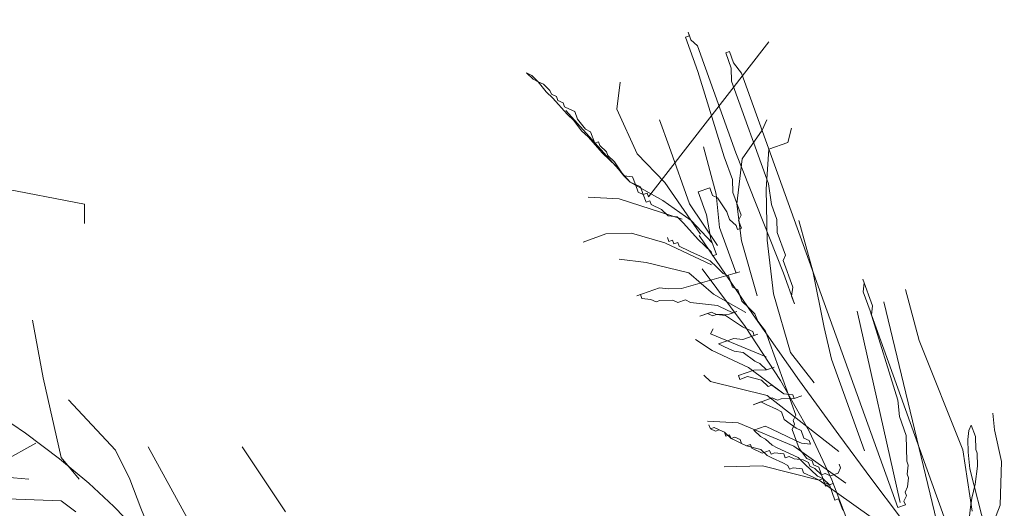
# Model space of a CAD drawing. Units: millimetres. Extents: x 595116 to 630915, y 909473 to 920225.
# Tile 23 of 134: x 629599.598 to 629606.562, y 919177.315 to 919180.767. Entities that reach past the tile are written whole.
import ezdxf

# ---------------------------------------------------------------- set-up
doc = ezdxf.new("R2010")
doc.units = ezdxf.units.MM
doc.layers.add('Dimension', color=3, linetype='Continuous', lineweight=18)
doc.layers.add('L-PLNT', color=85, linetype='Continuous', lineweight=13)
doc.styles.get("Standard").update_dxf_attribs({"font": 'arial.ttf'})
doc.dimstyles.new('ISO-25', dxfattribs={"dimtxt": 9, "dimasz": 6, "dimexe": 1.25, "dimexo": 0.625, "dimtad": 1, "dimlunit": 4, "dimtxsty": 'Standard', "dimcen": 2.5, "dimadec": 0, "dimazin": 0, "dimtfac": 1, "dimtmove": 0, "dimatfit": 3, "dimfxl": 1, "dimarcsym": 0})

# ---------------------------------------------------------------- blocks, each defined once
blk = doc.blocks.new('A$C143125F4')
for p, q in [((4.89065, 2.30713), (4.98365, 2.28921)), ((4.98365, 2.28921), (4.98365, 2.27577))]:
    blk.add_line(p, q)
blk = doc.blocks.new('A$C4FB75ABC')
for p, q in [((2.2354, 4.7176), (2.2283, 4.715)), ((2.2283, 4.715), (2.2515, 4.6504)), ((2.238, 4.7104), (2.2329, 4.7248)), ((2.2329, 4.7248), (2.2354, 4.7176)), ((2.1583, 4.4143), (2.3852, 4.7066)), ((2.2504, 4.6987), (2.238, 4.7104)), ((2.3227, 4.4977), (2.2504, 4.6987)), ((2.3109, 4.688), (2.3037, 4.6854)), ((2.3037, 4.6854), (2.314, 4.6567)), ((2.3186, 4.6665), (2.3109, 4.688)), ((2.3336, 4.6475), (2.3186, 4.6665)), ((1.9382, 4.6431), (1.9285, 4.6477)), ((1.9285, 4.6477), (1.9408, 4.6359)), ((1.9506, 4.6313), (1.9382, 4.6431)), ((2.2515, 4.6504), (2.3011, 4.49)), ((2.314, 4.6567), (2.3146, 4.6326)), ((2.6279, 3.8295), (2.3336, 4.6475)), ((1.9408, 4.6359), (1.9506, 4.6313)), ((1.9603, 4.6267), (1.9506, 4.6313)), ((1.9506, 4.6313), (1.9655, 4.6124)), ((1.9726, 4.6149), (1.9603, 4.6267)), ((2.0989, 4.5793), (2.1049, 4.6301)), ((2.3146, 4.6326), (2.3843, 4.4389)), ((1.9655, 4.6124), (1.9778, 4.6006)), ((1.9752, 4.6078), (1.9726, 4.6149)), ((1.985, 4.6032), (1.9752, 4.6078)), ((1.9876, 4.596), (1.985, 4.6032)), ((1.9778, 4.6006), (2.0051, 4.5699)), ((1.9973, 4.5914), (1.9876, 4.596)), ((1.9999, 4.5842), (1.9973, 4.5914)), ((2.0097, 4.5796), (1.9999, 4.5842)), ((2.1238, 4.4424), (2.0025, 4.577)), ((2.0051, 4.5699), (2.0174, 4.5581)), ((2.0194, 4.575), (2.0097, 4.5796)), ((2.0246, 4.5607), (2.0194, 4.575)), ((2.137, 4.4958), (2.0989, 4.5793)), ((2.0174, 4.5581), (2.0323, 4.5391)), ((2.0395, 4.5417), (2.0246, 4.5607)), ((2.197, 4.5092), (2.1789, 4.5595)), ((2.3723, 4.5399), (2.3815, 4.5594)), ((2.0323, 4.5391), (2.0447, 4.5274)), ((2.0493, 4.5371), (2.0395, 4.5417)), ((2.0447, 4.5274), (2.0719, 4.4967)), ((2.057, 4.5156), (2.0493, 4.5371)), ((2.335, 4.486), (2.3723, 4.5399)), ((2.4211, 4.5169), (2.4277, 4.5436)), ((2.0642, 4.5182), (2.057, 4.5156)), ((2.0668, 4.511), (2.0642, 4.5182)), ((2.0791, 4.4992), (2.0668, 4.511)), ((2.2357, 4.4016), (2.197, 4.5092)), ((2.3852, 4.504), (2.4211, 4.5169)), ((2.0719, 4.4967), (2.0966, 4.4731)), ((2.0817, 4.4921), (2.0791, 4.4992)), ((2.094, 4.4803), (2.0817, 4.4921)), ((2.189, 4.4415), (2.137, 4.4958)), ((2.2859, 4.4197), (2.2621, 4.5084)), ((2.3011, 4.49), (2.3166, 4.4469)), ((2.4125, 4.2707), (2.3227, 4.4977)), ((2.3797, 4.4291), (2.3852, 4.504)), ((2.1115, 4.4542), (2.094, 4.4803)), ((2.0966, 4.4731), (2.1115, 4.4542)), ((2.325, 4.4013), (2.335, 4.486)), ((2.1238, 4.4424), (2.1115, 4.4542)), ((2.1115, 4.4542), (2.1284, 4.4522)), ((2.1336, 4.4378), (2.1238, 4.4424)), ((2.185, 4.4077), (2.1238, 4.4424)), ((2.1284, 4.4522), (2.1336, 4.4378)), ((2.1388, 4.4235), (2.1336, 4.4378)), ((2.1336, 4.4378), (2.1434, 4.4332)), ((2.2564, 4.3442), (2.189, 4.4415)), ((2.3166, 4.4469), (2.3172, 4.4228)), ((2.3843, 4.4389), (2.3901, 4.4004)), ((2.1485, 4.4189), (2.1388, 4.4235)), ((2.1434, 4.4332), (2.1485, 4.4189)), ((2.1485, 4.4189), (2.1557, 4.4214)), ((2.1537, 4.4045), (2.1485, 4.4189)), ((2.1557, 4.4214), (2.1583, 4.4143)), ((2.2736, 4.4314), (2.2521, 4.4237)), ((2.2521, 4.4237), (2.2676, 4.3807)), ((2.2788, 4.4171), (2.2736, 4.4314)), ((2.2885, 4.4125), (2.2788, 4.4171)), ((2.2922, 4.3571), (2.2859, 4.4197)), ((2.3172, 4.4228), (2.3327, 4.3798)), ((2.382, 4.3327), (2.3797, 4.4291)), ((2.1029, 4.4105), (2.0449, 4.414)), ((2.222, 4.3723), (2.1029, 4.4105)), ((2.1609, 4.4071), (2.1537, 4.4045)), ((2.1634, 4.3999), (2.1609, 4.4071)), ((2.1829, 4.3907), (2.1634, 4.3999)), ((2.2389, 4.3703), (2.185, 4.4077)), ((2.2882, 4.3232), (2.2357, 4.4016)), ((2.306, 4.3864), (2.2885, 4.4125)), ((2.3338, 4.3316), (2.325, 4.4013)), ((2.3901, 4.4004), (2.4004, 4.3717)), ((2.1953, 4.379), (2.1829, 4.3907)), ((2.2122, 4.3769), (2.1953, 4.379)), ((2.2676, 4.3807), (2.2759, 4.335)), ((2.3112, 4.372), (2.306, 4.3864)), ((2.3327, 4.3798), (2.3281, 4.37)), ((2.2245, 4.3652), (2.2122, 4.3769)), ((2.2518, 4.3344), (2.2245, 4.3652)), ((2.2785, 4.3278), (2.2389, 4.3703)), ((2.3235, 4.3603), (2.3112, 4.372)), ((2.3261, 4.3531), (2.3235, 4.3603)), ((2.3281, 4.37), (2.3333, 4.3557)), ((2.4004, 4.3717), (2.401, 4.3476)), ((2.4678, 4.2744), (2.4414, 4.3703)), ((2.0779, 4.3448), (2.0349, 4.3293)), ((2.1261, 4.346), (2.0779, 4.3448)), ((2.1893, 4.3282), (2.1261, 4.346)), ((2.2538, 4.3417), (2.3557, 4.1924)), ((2.3232, 4.271), (2.2922, 4.3571)), ((2.3333, 4.3557), (2.3261, 4.3531)), ((2.401, 4.3476), (2.4165, 4.3046)), ((2.277, 4.2868), (2.1893, 4.3282)), ((2.1938, 4.3379), (2.1964, 4.3307)), ((2.1964, 4.3307), (2.2036, 4.3333)), ((2.2036, 4.3333), (2.2062, 4.3261)), ((2.2062, 4.3261), (2.2134, 4.3287)), ((2.2134, 4.3287), (2.2159, 4.3215)), ((2.2641, 4.3227), (2.2518, 4.3344)), ((2.2759, 4.335), (2.2862, 4.3063)), ((2.3628, 4.2285), (2.3338, 4.3316)), ((2.3941, 4.2317), (2.382, 4.3327)), ((2.2159, 4.3215), (2.2354, 4.3124)), ((2.2354, 4.3124), (2.2452, 4.3078)), ((2.2452, 4.3078), (2.255, 4.3032)), ((2.2765, 4.3109), (2.2641, 4.3227)), ((2.2791, 4.3037), (2.2765, 4.3109)), ((2.2862, 4.3063), (2.2791, 4.3037)), ((2.4165, 4.3046), (2.4119, 4.2948)), ((2.154, 4.2911), (2.1032, 4.2972)), ((2.234, 4.2713), (2.154, 4.2911)), ((2.255, 4.3032), (2.2745, 4.294)), ((2.2745, 4.294), (2.2868, 4.2822)), ((2.4119, 4.2948), (2.43, 4.2446)), ((2.2202, 4.242), (2.3304, 4.2736)), ((2.2808, 4.2314), (2.234, 4.2713)), ((2.3407, 4.1707), (2.2593, 4.2788)), ((2.2868, 4.2822), (2.2991, 4.2704)), ((2.2991, 4.2704), (2.3089, 4.2658)), ((2.4331, 4.2133), (2.4125, 4.2707)), ((2.4896, 4.1688), (2.4678, 4.2744)), ((2.3089, 4.2658), (2.3166, 4.2443)), ((2.5803, 4.2095), (2.5622, 4.2597)), ((2.5622, 4.2597), (2.5648, 4.2526)), ((2.5648, 4.2526), (2.5628, 4.2356)), ((2.1362, 4.228), (2.1792, 4.2435)), ((2.1434, 4.2306), (2.1362, 4.228)), ((2.1459, 4.2234), (2.1434, 4.2306)), ((2.1792, 4.2435), (2.1961, 4.2415)), ((2.1961, 4.2415), (2.2202, 4.242)), ((2.3419, 4.1967), (2.2808, 4.2314)), ((2.3166, 4.2443), (2.3264, 4.2397)), ((2.3264, 4.2397), (2.3341, 4.2182)), ((2.4257, 4.1214), (2.3941, 4.2317)), ((2.43, 4.2446), (2.4279, 4.2276)), ((2.5628, 4.2356), (2.5757, 4.1997)), ((2.6686, 4.144), (2.6423, 4.2399)), ((2.1629, 4.2214), (2.1459, 4.2234)), ((2.1726, 4.2168), (2.1629, 4.2214)), ((2.1798, 4.2194), (2.1726, 4.2168)), ((2.2039, 4.22), (2.1798, 4.2194)), ((2.2136, 4.2154), (2.2039, 4.22)), ((2.228, 4.2205), (2.2136, 4.2154)), ((2.2377, 4.2159), (2.228, 4.2205)), ((2.2716, 4.2119), (2.2377, 4.2159)), ((2.2885, 4.2099), (2.2716, 4.2119)), ((2.3341, 4.2182), (2.3465, 4.2064)), ((2.4279, 4.2276), (2.4331, 4.2133)), ((2.7169, 3.7399), (2.6018, 4.2172)), ((2.2552, 4.1898), (2.2768, 4.1975)), ((2.2696, 4.195), (2.2552, 4.1898)), ((2.2793, 4.1904), (2.2696, 4.195)), ((2.2768, 4.1975), (2.2865, 4.1929)), ((2.2865, 4.1929), (2.3106, 4.1935)), ((2.308, 4.2007), (2.2885, 4.2099)), ((2.3178, 4.1961), (2.308, 4.2007)), ((2.3106, 4.1935), (2.325, 4.1987)), ((2.325, 4.1987), (2.3178, 4.1961)), ((2.3465, 4.2064), (2.3588, 4.1946)), ((2.3588, 4.1946), (2.364, 4.1803)), ((2.6325, 3.8393), (2.5516, 4.1992)), ((2.5757, 4.1997), (2.6279, 4.0321)), ((2.5783, 4.1926), (2.5803, 4.2095)), ((0.9973, 4.1826), (1.0177, 4.0736)), ((2.2865, 4.1929), (2.2793, 4.1904)), ((2.3034, 4.1909), (2.2865, 4.1929)), ((2.3353, 4.17), (2.3034, 4.1909)), ((2.3557, 4.1924), (2.443, 4.0685)), ((2.364, 4.1803), (2.3789, 4.1614)), ((2.8029, 3.5683), (2.5783, 4.1926)), ((2.2753, 4.1565), (2.2799, 4.1663)), ((2.38, 4.1131), (2.2753, 4.1565)), ((2.345, 4.1654), (2.3353, 4.17)), ((2.3359, 4.1459), (2.3645, 4.1562)), ((2.4072, 4.0691), (2.3407, 4.1707)), ((2.3548, 4.1608), (2.345, 4.1654)), ((2.3574, 4.1536), (2.3548, 4.1608)), ((2.3645, 4.1562), (2.3574, 4.1536)), ((2.3789, 4.1614), (2.4357, 4.0035)), ((2.5031, 4.1088), (2.4896, 4.1688)), ((2.2785, 4.1252), (2.2466, 4.1462)), ((2.2902, 4.1376), (2.3189, 4.1479)), ((2.3, 4.133), (2.2902, 4.1376)), ((2.3189, 4.1479), (2.3359, 4.1459)), ((2.7507, 3.9385), (2.6686, 4.144)), ((2.3468, 4.0931), (2.2785, 4.1252)), ((2.3098, 4.1284), (2.3, 4.133)), ((2.3195, 4.1238), (2.3098, 4.1284)), ((2.3364, 4.1218), (2.3195, 4.1238)), ((2.3585, 4.1054), (2.3364, 4.1218)), ((2.4704, 4.0646), (2.4257, 4.1214)), ((2.3683, 4.1008), (2.3585, 4.1054)), ((2.3806, 4.089), (2.3683, 4.1008)), ((2.5651, 3.9366), (2.5031, 4.1088)), ((2.3278, 4.0781), (2.3565, 4.0885)), ((2.413, 4.044), (2.3468, 4.0931)), ((2.3565, 4.0885), (2.3806, 4.089)), ((2.3806, 4.089), (2.395, 4.0942)), ((2.395, 4.0942), (2.3806, 4.089)), ((1.0177, 4.0736), (1.0518, 3.9238)), ((2.275, 4.0672), (2.2627, 4.079)), ((2.3818, 4.0408), (2.275, 4.0672)), ((2.3304, 4.071), (2.3278, 4.0781)), ((2.3448, 4.0761), (2.3304, 4.071)), ((2.3714, 4.0695), (2.3448, 4.0761)), ((2.3838, 4.0577), (2.3714, 4.0695)), ((2.4608, 3.9732), (2.4072, 4.0691)), ((2.443, 4.0685), (2.5171, 3.9664)), ((2.3909, 4.0603), (2.3838, 4.0577)), ((2.413, 4.044), (2.3909, 4.0603)), ((1.0654, 4.0327), (1.154, 3.9374)), ((2.3557, 4.0233), (2.3915, 4.0362)), ((2.37, 4.0285), (2.3557, 4.0233)), ((2.3798, 4.0239), (2.37, 4.0285)), ((2.5169, 3.9354), (2.3818, 4.0408)), ((2.3915, 4.0362), (2.4013, 4.0316)), ((2.4013, 4.0316), (2.4084, 4.0342)), ((2.4084, 4.0342), (2.4325, 4.0348)), ((2.43, 4.0419), (2.413, 4.044)), ((2.4325, 4.0348), (2.43, 4.0419)), ((2.4325, 4.0348), (2.4469, 4.0399)), ((2.4469, 4.0399), (2.4325, 4.0348)), ((2.6279, 4.0321), (2.6311, 4.0008)), ((0.9842, 3.9699), (0.9085, 4.0207)), ((2.3993, 4.0147), (2.3798, 4.0239)), ((2.409, 4.0101), (2.3993, 4.0147)), ((2.4142, 3.9957), (2.409, 4.0101)), ((2.3275, 3.9889), (2.2696, 3.9923)), ((2.4363, 3.9794), (2.4142, 3.9957)), ((2.4357, 4.0035), (2.4311, 3.9937)), ((2.4311, 3.9937), (2.4337, 3.9866)), ((2.6311, 4.0008), (2.644, 3.965)), ((2.8101, 3.9761), (2.8069, 4.0074)), ((2.2748, 3.978), (2.2722, 3.9852)), ((2.2722, 3.9852), (2.2748, 3.978)), ((2.2748, 3.978), (2.2819, 3.9806)), ((2.2845, 3.9734), (2.2748, 3.978)), ((2.2819, 3.9806), (2.2917, 3.976)), ((2.2917, 3.976), (2.2845, 3.9734)), ((2.3014, 3.9714), (2.2917, 3.976)), ((2.2917, 3.976), (2.3014, 3.9714)), ((2.304, 3.9642), (2.3014, 3.9714)), ((2.3014, 3.9714), (2.3138, 3.9596)), ((2.4323, 3.9455), (2.3275, 3.9889)), ((2.3568, 3.9751), (2.3783, 3.9828)), ((2.3691, 3.9633), (2.3568, 3.9751)), ((2.3783, 3.9828), (2.3881, 3.9782)), ((2.3881, 3.9782), (2.4076, 3.9691)), ((2.4337, 3.9866), (2.4291, 3.9768)), ((2.4291, 3.9768), (2.442, 3.9409)), ((2.446, 3.9748), (2.4363, 3.9794)), ((2.4512, 3.9604), (2.446, 3.9748)), ((2.5035, 3.8821), (2.4608, 3.9732)), ((2.7619, 3.975), (2.7599, 3.958)), ((2.7665, 3.9847), (2.7619, 3.975)), ((2.7742, 3.9632), (2.7665, 3.9847)), ((2.8236, 3.9161), (2.8101, 3.9761)), ((1.0487, 3.9217), (0.9842, 3.9699)), ((2.3112, 3.9668), (2.304, 3.9642)), ((2.3138, 3.9596), (2.3112, 3.9668)), ((2.3209, 3.9622), (2.3138, 3.9596)), ((2.3138, 3.9596), (2.3235, 3.955)), ((2.3307, 3.9576), (2.3209, 3.9622)), ((2.3235, 3.955), (2.3333, 3.9504)), ((2.3333, 3.9504), (2.3307, 3.9576)), ((2.3789, 3.9587), (2.3691, 3.9633)), ((2.3912, 3.947), (2.3789, 3.9587)), ((2.4076, 3.9691), (2.4173, 3.9645)), ((2.4173, 3.9645), (2.4368, 3.9553)), ((2.4368, 3.9553), (2.4466, 3.9507)), ((2.4609, 3.9558), (2.4512, 3.9604)), ((2.4635, 3.9487), (2.4609, 3.9558)), ((2.5171, 3.9664), (2.5794, 3.8826)), ((2.644, 3.965), (2.6451, 3.9167)), ((2.7599, 3.958), (2.7605, 3.9339)), ((2.7748, 3.9391), (2.7742, 3.9632)), ((1.0041, 3.951), (0.9428, 3.917)), ((1.154, 3.9374), (1.1812, 3.8829)), ((1.2153, 3.9442), (1.2902, 3.808)), ((1.3924, 3.9442), (1.4742, 3.8217)), ((2.343, 3.9458), (2.3333, 3.9504)), ((2.3333, 3.9504), (2.343, 3.9458)), ((2.3502, 3.9484), (2.343, 3.9458)), ((2.343, 3.9458), (2.3697, 3.9392)), ((2.3528, 3.9412), (2.3502, 3.9484)), ((2.3723, 3.932), (2.3528, 3.9412)), ((2.3697, 3.9392), (2.3821, 3.9274)), ((2.3866, 3.9372), (2.3723, 3.932)), ((2.3892, 3.93), (2.3866, 3.9372)), ((2.401, 3.9424), (2.3912, 3.947)), ((2.44, 3.924), (2.401, 3.9424)), ((2.5304, 3.8755), (2.4323, 3.9455)), ((2.442, 3.9409), (2.4569, 3.922)), ((2.4466, 3.9507), (2.4635, 3.9487)), ((2.7679, 3.8231), (2.7507, 3.9385)), ((2.7605, 3.9339), (2.7636, 3.9026)), ((2.7774, 3.9319), (2.7748, 3.9391)), ((1.1035, 3.8758), (1.0487, 3.9217)), ((1.0518, 3.9238), (1.0858, 3.8829)), ((2.3821, 3.9274), (2.3918, 3.9228)), ((2.3964, 3.9326), (2.3892, 3.93)), ((2.3918, 3.9228), (2.4113, 3.9137)), ((2.4133, 3.9306), (2.3964, 3.9326)), ((2.4159, 3.9234), (2.4133, 3.9306)), ((2.4231, 3.926), (2.4159, 3.9234)), ((2.4328, 3.9214), (2.4231, 3.926)), ((2.4498, 3.9194), (2.4328, 3.9214)), ((2.4523, 3.9122), (2.44, 3.924)), ((2.4595, 3.9148), (2.4498, 3.9194)), ((2.4569, 3.922), (2.4667, 3.9174)), ((2.4621, 3.9076), (2.4595, 3.9148)), ((2.4667, 3.9174), (2.4693, 3.9102)), ((2.6451, 3.9167), (2.6477, 3.9096)), ((2.778, 3.9078), (2.7774, 3.9319)), ((2.8207, 3.834), (2.8236, 3.9161)), ((2.3729, 3.9079), (2.3006, 3.9062)), ((2.4796, 3.8815), (2.3729, 3.9079)), ((2.4113, 3.9137), (2.4211, 3.9091)), ((2.4211, 3.9091), (2.4237, 3.9019)), ((2.4237, 3.9019), (2.4308, 3.9045)), ((2.4308, 3.9045), (2.4478, 3.9025)), ((2.4478, 3.9025), (2.4503, 3.8953)), ((2.477, 3.8887), (2.4523, 3.9122)), ((2.4718, 3.903), (2.4621, 3.9076)), ((2.4693, 3.9102), (2.479, 3.9056)), ((2.4842, 3.8913), (2.4718, 3.903)), ((2.479, 3.9056), (2.4868, 3.8841)), ((2.52, 3.9042), (2.5155, 3.8944)), ((2.5175, 3.9113), (2.52, 3.9042)), ((2.6477, 3.9096), (2.6457, 3.8926)), ((2.7636, 3.9026), (2.8247, 3.6653)), ((2.7739, 3.8739), (2.778, 3.9078)), ((0.9905, 3.8829), (0.9155, 3.8897)), ((1.1812, 3.8829), (1.2017, 3.8285)), ((2.4503, 3.8953), (2.4698, 3.8861)), ((2.4698, 3.8861), (2.4796, 3.8815)), ((2.4868, 3.8841), (2.477, 3.8887)), ((2.4796, 3.8815), (2.4868, 3.8841)), ((2.5777, 3.8114), (2.4796, 3.8815)), ((2.4914, 3.8938), (2.4842, 3.8913)), ((2.4868, 3.8841), (2.4893, 3.8769)), ((2.4919, 3.8697), (2.4868, 3.8841)), ((2.4868, 3.8841), (2.4991, 3.8723)), ((2.5011, 3.8892), (2.4914, 3.8938)), ((2.5155, 3.8944), (2.5011, 3.8892)), ((2.5372, 3.7949), (2.5035, 3.8821)), ((2.5794, 3.8826), (2.6314, 3.8136)), ((2.6457, 3.8926), (2.6483, 3.8855)), ((2.6483, 3.8855), (2.6463, 3.8685)), ((1.1506, 3.8319), (1.1035, 3.8758)), ((2.4893, 3.8769), (2.4991, 3.8723)), ((2.5063, 3.8749), (2.4919, 3.8697)), ((2.4991, 3.8723), (2.5063, 3.8749)), ((2.4991, 3.8723), (2.5094, 3.8436)), ((2.6463, 3.8685), (2.6417, 3.8588)), ((2.7673, 3.8473), (2.7739, 3.8739)), ((0.8746, 3.8489), (1.0518, 3.8421)), ((1.0518, 3.8421), (1.079, 3.8217)), ((2.5094, 3.8436), (2.5166, 3.8462)), ((2.5166, 3.8462), (2.5244, 3.8247)), ((2.6443, 3.8516), (2.6397, 3.8418)), ((2.6397, 3.8418), (2.6423, 3.8347)), ((2.6417, 3.8588), (2.6443, 3.8516)), ((2.7653, 3.8303), (2.7673, 3.8473)), ((1.1917, 3.7897), (1.1506, 3.8319)), ((1.2017, 3.8285), (1.2153, 3.7944)), ((2.6423, 3.8347), (2.6279, 3.8295)), ((2.7613, 3.7965), (2.7653, 3.8303)), ((2.7957, 3.7683), (2.8207, 3.834))]:
    blk.add_line(p, q)
blk = doc.blocks.new('*D216')
at = {"layer": 'Defpoints', "color": 0, "transparency": 16777216}
for p in [(629743.5408, 919411.9276), (629505.0408, 919411.8279), (629743.5408, 918832.3776)]:
    blk.add_point(p, dxfattribs=at)
at = {"layer": 'Dimension', "color": 0, "lineweight": -2, "transparency": 16777216}
for p, q in [((629743.5408, 919411.3026), (629743.5408, 918831.1276)), ((629505.0408, 919411.2029), (629505.0408, 918831.1276)), ((629511.0408, 918832.3776), (629737.5408, 918832.3776))]:
    blk.add_line(p, q, dxfattribs=at)
at = {"layer": 'Dimension', "color": 0, "transparency": 16777216}
for points in [[(629511.0408, 918833.3776), (629511.0408, 918831.3776), (629505.0408, 918832.3776)], [(629737.5408, 918833.3776), (629737.5408, 918831.3776), (629743.5408, 918832.3776)]]:
    blk.add_solid(points, dxfattribs=at)
at = {"layer": 'Dimension', "color": 0, "transparency": 16777216, "insert": (629624.2908, 918837.656), "char_height": 9, "attachment_point": 5}
blk.add_mtext('19\'-10 1/2"', dxfattribs=at)

msp = doc.modelspace()

# ---------------------------------------------------------------- block references
at = {"layer": 'L-PLNT'}
for name, p, xscale, yscale, zscale in [('A$C143125F4', (629549.214, 919156.1107), 10.20167662382051, 10.20167662382051, 10.20167662382051), ('A$C4FB75ABC', (629595.9442, 919162.9458), 3.753413438031968, 3.753413438031968, 3.753413438031968)]:
    msp.add_blockref(name, p, dxfattribs=dict(at, xscale=xscale, yscale=yscale, zscale=zscale))

# ---------------------------------------------------------------- dimensions: what is measured, and where the dimension line sits
at = {"layer": 'Dimension'}
dim = msp.add_linear_dim(base=(629743.5408, 918832.3776), p1=(629505.0408, 919411.8279), p2=(629743.5408, 919411.9276), dimstyle='ISO-25', override={"dimdec": 1, "dimlfac": 1, "dimrnd": 0, "dimzin": 1, "dimdsep": 46, "dimlunit": 4, "dimfrac": 2}, dxfattribs=at)
dim.commit()
dim.dimension.update_dxf_attribs({"geometry": '*D216', "text_midpoint": (629624.2908, 918837.656)})

doc.saveas('drawing.dxf')
